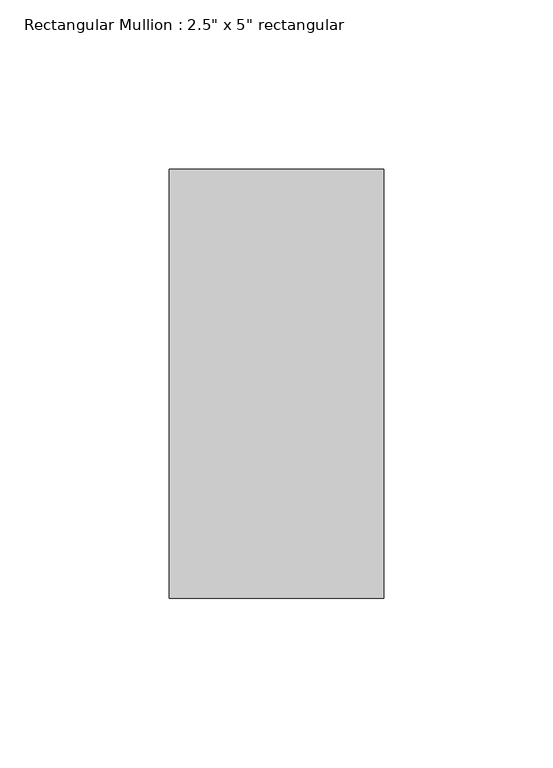
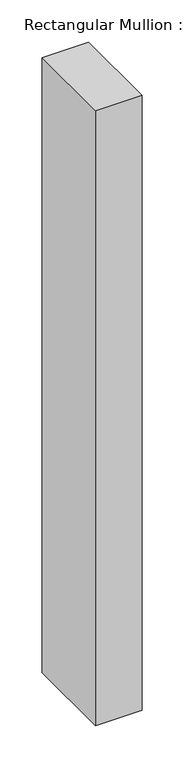
"""IFC4 building model written with IfcOpenShell, lengths in millimetres: member geometry."""

from ifc_helpers import new_model, si_unit, frame, origin, place, context, project, spatial, polyline, outline, extrude, source, transform, mapped, element, save


def member_59fcad1a(model_context):
    return source(origin(), model_context, "Body", "SweptSolid", [
        extrude(outline(polyline([(0.0, 63.5), (0.0, -63.5), (-63.5, -63.5), (-63.5, 63.5), (0.0, 63.5)])), frame((0.0, 0.0, -889.8127727), z_axis=(0.0, 0.0, 1.0), x_axis=(1.0, 0.0, 0.0)), (0.0, 0.0, 1.0), 889.8127727),
    ])


if __name__ == "__main__":
    model = new_model("IFC4")
    model_context = context("Model", 3, world=origin())
    ifc_project = project(units=[si_unit("LENGTHUNIT", "METRE", prefix="MILLI")], contexts=[model_context])
    site = spatial("IfcSite", under=ifc_project)
    building = spatial("IfcBuilding", under=site)
    placement = place(None, origin())
    member_shape = member_59fcad1a(model_context)
    element("IfcMember", 1, ObjectType="Rectangular Mullion : 2.5\" x 5\" rectangular", at=placement, inside=building, context=model_context, shape_type="MappedRepresentation", body=[
        mapped(member_shape, transform((0.0, 0.0, 0.0), x_axis=(1.0, 0.0, 0.0), y_axis=(0.0, 1.0, 0.0), z_axis=(0.0, 0.0, 1.0))),
    ])
    save(model, "model.ifc")

# Revit data of these elements
# Type "Rectangular Mullion : 2.5\" x 5\" rectangular"
#   built-in parameter 1007304 = 0.416667 (stored number, unit not read)
#   built-in parameter 1007301 = 0.104167 (stored number, unit not read)
#   built-in parameter 1007300 = 0.104167 (stored number, unit not read)
# Element 1 (IfcMember, "Rectangular Mullion : 2.5\" x 5\" rectangular")
#   Materials on its faces: "Aluminum"
# Materials
#   "Aluminum": class "Metal", colour RGB 247 247 247, transparency 0, Description = "Aluminum 6061", Cost = 0
